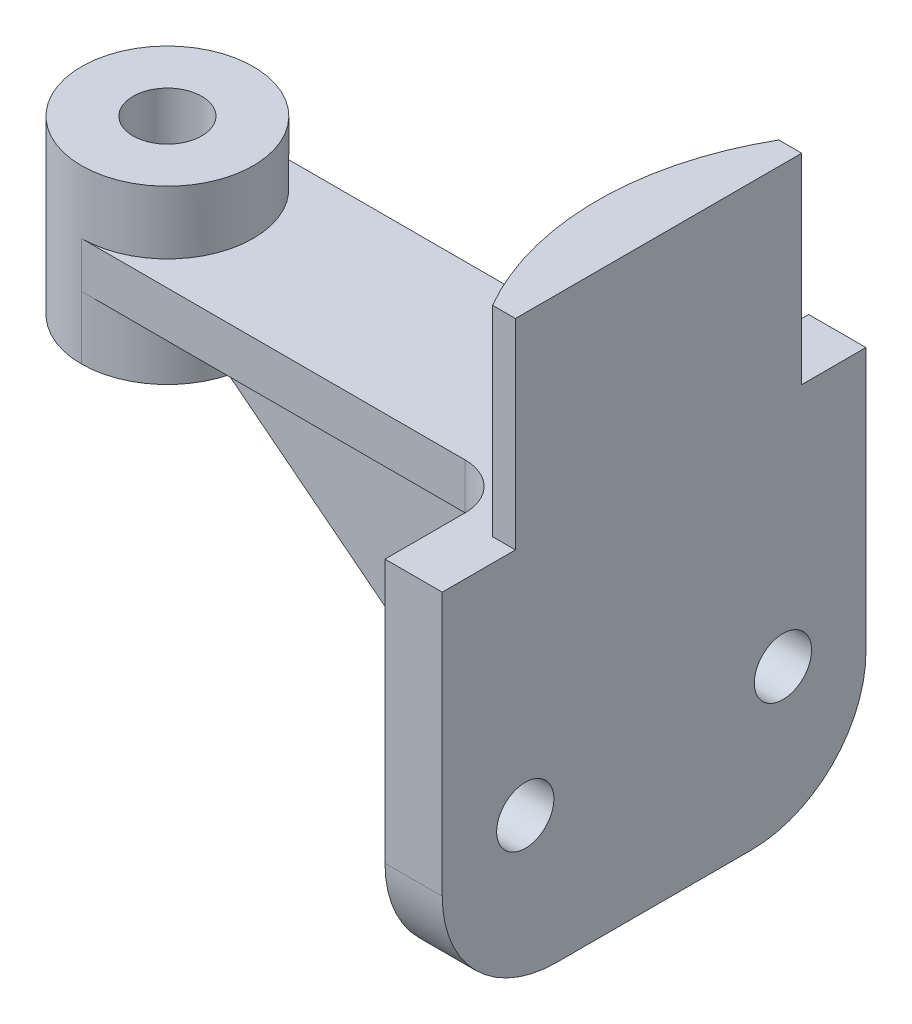
from build123d import *

# Parameters (mm, degrees)
HUB_PROFILE_R              = 15
HUB_30_DEPTH               = 30
BORE_PROFILE_R             = 6
BORE_12_DEPTH              = 60
ARM_DEPTH                  = 4
MOUNTING_PLATE_DEPTH       = 35
PLATE_LUG_DEPTH            = 10
MOUNTING_HOLES_PROFILE_R   = 5
MOUNTING_HOLES_2X_10_DEPTH = 87
SUPPORT_RIB_REACH          = 109.285
RIB_LINE_WALL_W            = 292.786132162
RIB_LINE_WALL_H            = 8


with BuildPart() as part:
    # Hub Profile → Hub Ø30 (new body)
    with BuildSketch(Plane(origin=(0, 0, 0), x_dir=(1, 0, 0), z_dir=(0, 1, 0))):
        with Locations(Location((0, 0, 0), (0, 0, 270))):
            Circle(HUB_PROFILE_R)
    extrude(amount=HUB_30_DEPTH)

    # Bore Profile → Bore Ø12 (cut)
    with BuildSketch(Plane(origin=(0, 30, 0), x_dir=(1, 0, 0), z_dir=(0, 1, 0))):
        with Locations(Location((0, 0, 0), (0, 0, 270))):
            Circle(BORE_PROFILE_R)
    extrude(amount=-BORE_12_DEPTH, mode=Mode.SUBTRACT)

    # Arm Profile → Arm (add, symmetric)
    with BuildSketch(Plane(origin=(0, 15, 0), x_dir=(1, 0, 0), z_dir=(0, 1, 0))):
        with BuildLine():
            Line((85, 0), (85, 37))
            Line((85, 37), (75, 37))
            Line((75, 37), (75, 23))
            ThreePointArc((75, 23), (72.656854249, 17.343145751), (67, 15))
            Line((67, 15), (0, 15))
            ThreePointArc((0, 15), (15, 0), (0, -15))
            Line((0, -15), (67, -15))
            ThreePointArc((67, -15), (72.656854249, -17.343145751), (75, -23))
            Line((75, -23), (75, -37))
            Line((75, -37), (85, -37))
            Line((85, -37), (85, 0))
        make_face()
    extrude(amount=ARM_DEPTH, both=True)

    # Mounting Plate Profile → Mounting Plate (add)
    with BuildSketch(Plane(origin=(0, 19, 0), x_dir=(1, 0, 0), z_dir=(0, 1, 0))):
        with BuildLine():
            Line((85, 0.780866297), (85, 25.780866297))
            Line((85, 25.780866297), (81, 25.780866297))
            ThreePointArc((81, 25.780866297), (74.301270189, 0.780866297), (81, -24.219133703))
            Line((81, -24.219133703), (85, -24.219133703))
            Line((85, -24.219133703), (85, 0.780866297))
        make_face()
    extrude(amount=MOUNTING_PLATE_DEPTH)

    # Plate Lug Profile → Plate Lug (add)
    with BuildSketch(Plane(origin=(85, 0, 0), x_dir=(0, 0, -1), z_dir=(1, 0, 0))):
        with BuildLine():
            Line((-37, 11), (-37, -27))
            ThreePointArc((-37, -27), (-31.142135624, -41.142135624), (-17, -47))
            Line((-17, -47), (17, -47))
            ThreePointArc((17, -47), (31.142135624, -41.142135624), (37, -27))
            Line((37, -27), (37, 11))
            Line((37, 11), (-37, 11))
        make_face()
    extrude(amount=-PLATE_LUG_DEPTH)

    # Mounting Holes Profile → Mounting Holes 2xØ10 (cut)
    with BuildSketch(Plane(origin=(85, 0, 0), x_dir=(0, 0, -1), z_dir=(1, 0, 0))):
        with Locations((22.5, -22)):
            Circle(MOUNTING_HOLES_PROFILE_R)
        with Locations((-22.5, -22)):
            Circle(MOUNTING_HOLES_PROFILE_R)
    extrude(amount=-MOUNTING_HOLES_2X_10_DEPTH, mode=Mode.SUBTRACT)

    # Rib Line wall → Support Rib (add, up to next)
    with BuildSketch(Plane(origin=(45, -23.5, 0), x_dir=(0.787228053529, -0.616661975264, 0), z_dir=(0.616661975264, 0.787228053529, 0)), mode=Mode.PRIVATE) as support_rib_sk1:
        Rectangle(RIB_LINE_WALL_W, RIB_LINE_WALL_H)
    support_rib_tool1 = extrude(support_rib_sk1.sketch, amount=SUPPORT_RIB_REACH, mode=Mode.PRIVATE) - part.part
    add(support_rib_tool1.solids().sort_by_distance((45, -23.5, 0))[0])


solid = part.part
